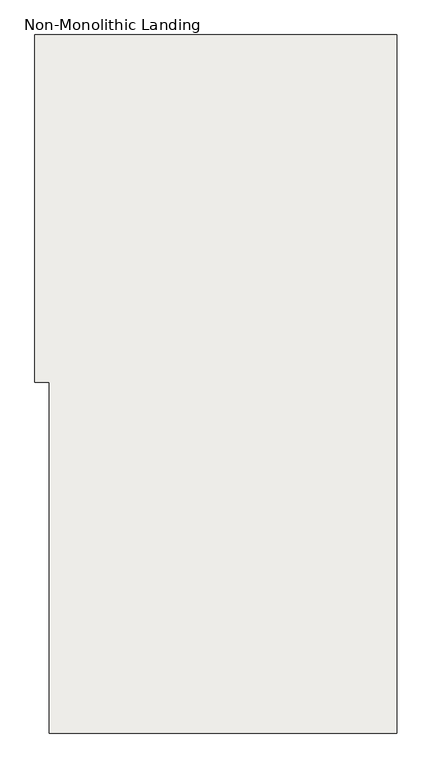
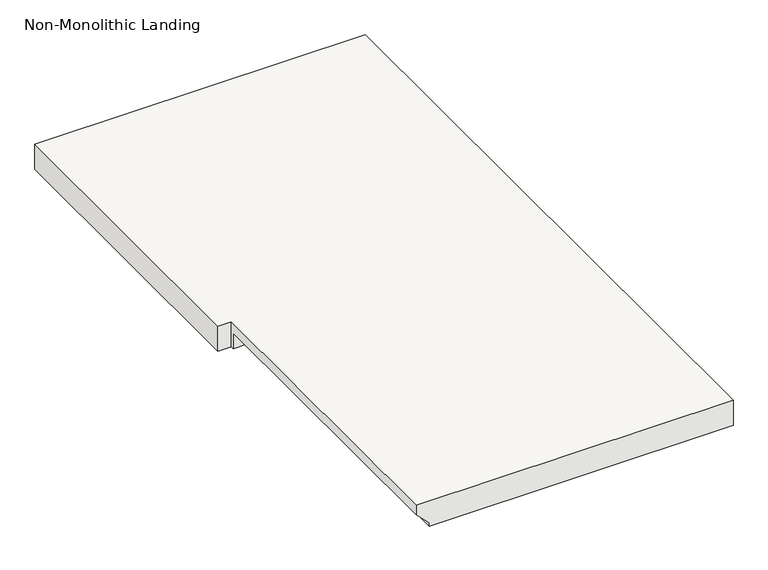
"""IFC4 building model written with IfcOpenShell, lengths in millimetres: slab geometry, Non-Monolithic Landing."""

from ifc_helpers import new_model, si_unit, origin, place, context, project, spatial, faceted_brep, source, transform, mapped, element, save


def non_monolithic_landing_6134172e(model_context):
    return source(origin(), model_context, "Body", "Brep", [
        faceted_brep([(-2686.3634065, 3724.7702159, 8001.0), (-2686.3634065, 4950.530501, 8001.0), (-3295.9634065, 4950.530501, 8001.0), (-3321.3634065, 4950.530501, 8001.0), (-3321.3634065, 4340.930501, 8001.0), (-3295.9634065, 4340.930501, 8001.0), (-3295.9634065, 3724.7702159, 8001.0), (-3270.5634065, 4334.3702159, 7950.2), (-3295.9634065, 4334.3702159, 7950.2), (-3295.9634065, 4340.930501, 7950.2), (-3321.3634065, 4340.930501, 7950.2), (-3321.3634065, 4950.530501, 7950.2), (-3295.9634065, 4950.530501, 7950.2), (-2686.3634065, 4950.530501, 7950.2), (-2686.3634065, 3724.7702159, 7950.2), (-3270.5634065, 3724.7702159, 7950.2), (-3295.9634065, 4334.3702159, 7981.95), (-3295.9634065, 3724.7702159, 7981.95), (-3270.5634065, 3724.7702159, 7956.55), (-3270.5634065, 4334.3702159, 7956.55)], [[[0, 1, 2, 3, 4, 5, 6]], [[7, 8, 9, 10, 11, 12, 13, 14, 15]], [[2, 1, 13, 12]], [[4, 3, 11, 10]], [[3, 2, 12, 11]], [[6, 5, 9, 8, 16, 17]], [[0, 6, 17, 18, 15, 14]], [[18, 17, 16, 19]], [[8, 7, 19, 16]], [[7, 15, 18, 19]], [[1, 0, 14, 13]], [[5, 4, 10, 9]]]),
    ])


if __name__ == "__main__":
    model = new_model("IFC4")
    model_context = context("Model", 3, world=origin())
    ifc_project = project(units=[si_unit("LENGTHUNIT", "METRE", prefix="MILLI")], contexts=[model_context])
    site = spatial("IfcSite", under=ifc_project)
    building = spatial("IfcBuilding", under=site)
    placement = place(None, origin())
    non_monolithic_landing_shape = non_monolithic_landing_6134172e(model_context)
    element("IfcSlab", 1, ObjectType="Non-Monolithic Landing", at=placement, inside=building, context=model_context, shape_type="MappedRepresentation", body=[
        mapped(non_monolithic_landing_shape, transform((0.0, 0.0, 0.0), x_axis=(1.0, 0.0, 0.0), y_axis=(0.0, 1.0, 0.0), z_axis=(0.0, 0.0, 1.0))),
    ])
    save(model, "model.ifc")
